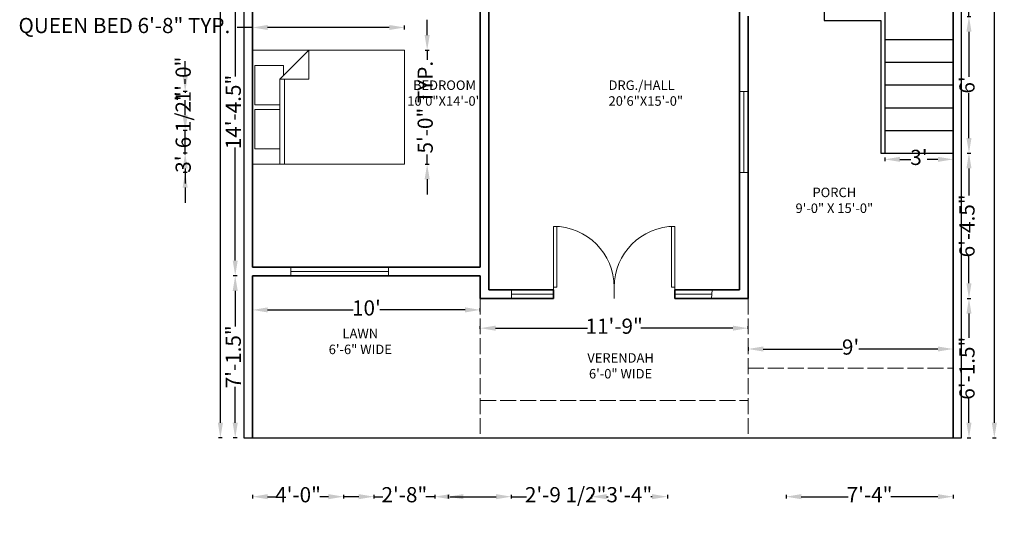
# Model space of a CAD drawing. Units: inches. Extents: x 2174 to 2692, y 577 to 1264.
# Tile 1 of 5: x 2174 to 2692, y 577 to 841. Entities that reach past the tile are written whole.
import ezdxf

# ---------------------------------------------------------------- set-up
doc = ezdxf.new("R2010")
doc.units = ezdxf.units.IN
doc.linetypes.add('ACAD_ISO02W100', pattern=[15, 12, -3])
for name, color, linetype, lineweight in [('A-ANNO-DIMS', 2, 'Continuous', 13), ('A-AREA-IDEN', 7, 'Continuous', 18), ('A-DOOR', 3, 'Continuous', 18), ('A-FLOR-EDGE', 8, 'ACAD_ISO02W100', 18), ('A-FLOR-STRS', 7, 'Continuous', 25), ('A-FURN', 8, 'Continuous', 18), ('A-GLAZ', 4, 'Continuous', 18), ('A-WALL', 7, 'Continuous', 35), ('C-PROP', 7, 'Continuous', 25)]:
    doc.layers.add(name, color=color, linetype=linetype, lineweight=lineweight)
doc.styles.get("Standard").update_dxf_attribs({"font": 'arial.ttf'})
doc.dimstyles.new('ISO-25', dxfattribs={"dimtxt": 8, "dimasz": 8, "dimexe": 1, "dimexo": 1, "dimtad": 0, "dimdec": 1, "dimlunit": 3, "dimtxsty": 'Standard', "dimcen": 2.5, "dimclrd": 1, "dimclre": 1, "dimclrt": 1, "dimadec": 0, "dimazin": 0, "dimtfac": 1, "dimtdec": 1, "dimtmove": 0, "dimatfit": 3, "dimfxl": 1, "dimfxlon": 1, "dimarcsym": 0})

# ---------------------------------------------------------------- blocks, each defined once
blk = doc.blocks.new('Bed - Queen')
for p, q in [((0, -80.00003), (0, 0)), ((0, 0), (59.99999, 0)), ((59.99999, 0), (59.99999, -80.00003)), ((7.99999, -1.2), (28.79998, -1.2)), ((7.99999, -14.4), (7.99999, -1.2)), ((28.79998, -1.2), (28.79998, -14.4)), ((31.19999, -1.2), (51.99999, -1.2)), ((31.19999, -14.4), (31.19999, -1.2)), ((51.99999, -1.2), (51.99999, -16.4)), ((0, -14.4), (44.8, -14.4)), ((59.99999, -29.6), (44.8, -14.4)), ((44.8, -14.4), (44.8, -29.6)), ((44.8, -16.8), (0, -16.8)), ((51.99999, -16.4), (46.79936, -16.4)), ((44.8, -29.6), (59.99999, -29.6)), ((59.99999, -80.00003), (0, -80.00003))]:
    blk.add_line(p, q)
blk = doc.blocks.new('*D15')
at = {"layer": 'A-ANNO-DIMS', "color": 0, "lineweight": -2, "transparency": 16777216}
for p, q in [((2629.45, 768.14), (2629.45, 766.14)), ((2665.45, 768.14), (2665.45, 766.14)), ((2637.45, 767.14), (2643.15, 767.14)), ((2657.45, 767.14), (2651.76, 767.14))]:
    blk.add_line(p, q, dxfattribs=at)
at = {"layer": 'A-ANNO-DIMS', "color": 0, "transparency": 16777216}
for points in [[(2637.45, 768.48), (2637.45, 765.81), (2629.45, 767.14)], [(2657.45, 768.48), (2657.45, 765.81), (2665.45, 767.14)]]:
    blk.add_solid(points, dxfattribs=at)
at = {"layer": 'Defpoints', "color": 0, "transparency": 16777216}
for p in [(2629.45, 770.35), (2665.45, 770.35), (2629.45, 767.14)]:
    blk.add_point(p, dxfattribs=at)
at = {"layer": 'A-ANNO-DIMS', "color": 0, "transparency": 16777216, "insert": (2647.45, 767.14), "char_height": 8, "attachment_point": 5}
blk.add_mtext("3'", dxfattribs=at)
blk = doc.blocks.new('*D16')
at = {"layer": 'A-ANNO-DIMS', "color": 0, "lineweight": -2, "transparency": 16777216}
for p, q in [((2296.45, 686.99), (2296.45, 688.82)), ((2304.45, 687.82), (2349.42, 687.82)), ((2408.45, 687.82), (2363.49, 687.82)), ((2416.45, 686.99), (2416.45, 688.82))]:
    blk.add_line(p, q, dxfattribs=at)
at = {"layer": 'A-ANNO-DIMS', "color": 0, "transparency": 16777216}
for points in [[(2304.45, 689.15), (2304.45, 686.48), (2296.45, 687.82)], [(2408.45, 689.15), (2408.45, 686.48), (2416.45, 687.82)]]:
    blk.add_solid(points, dxfattribs=at)
at = {"layer": 'Defpoints', "color": 0, "transparency": 16777216}
for p in [(2296.45, 685.99), (2416.45, 687.82), (2416.45, 685.99)]:
    blk.add_point(p, dxfattribs=at)
at = {"layer": 'A-ANNO-DIMS', "color": 0, "transparency": 16777216, "insert": (2356.45, 687.82), "char_height": 8, "attachment_point": 5}
blk.add_mtext("10'", dxfattribs=at)
blk = doc.blocks.new('*D17')
at = {"layer": 'A-ANNO-DIMS', "color": 0, "lineweight": -2, "transparency": 16777216}
for p, q in [((2416.45, 677.83), (2416.45, 679.2)), ((2424.45, 678.2), (2472.96, 678.2)), ((2549.45, 678.2), (2500.94, 678.2)), ((2557.45, 677.83), (2557.45, 679.2))]:
    blk.add_line(p, q, dxfattribs=at)
at = {"layer": 'A-ANNO-DIMS', "color": 0, "transparency": 16777216}
for points in [[(2424.45, 679.53), (2424.45, 676.87), (2416.45, 678.2)], [(2549.45, 679.53), (2549.45, 676.87), (2557.45, 678.2)]]:
    blk.add_solid(points, dxfattribs=at)
at = {"layer": 'Defpoints', "color": 0, "transparency": 16777216}
for p in [(2416.45, 676.83), (2557.45, 678.2), (2557.45, 676.83)]:
    blk.add_point(p, dxfattribs=at)
at = {"layer": 'A-ANNO-DIMS', "color": 0, "transparency": 16777216, "insert": (2486.95, 678.2), "char_height": 8, "attachment_point": 5}
blk.add_mtext('11\'-9"', dxfattribs=at)
blk = doc.blocks.new('*D18')
at = {"layer": 'A-ANNO-DIMS', "color": 0, "lineweight": -2, "transparency": 16777216}
for p, q in [((2557.45, 668.21), (2557.45, 666.21)), ((2565.45, 667.21), (2607.15, 667.21)), ((2657.45, 667.21), (2615.76, 667.21)), ((2665.45, 668.21), (2665.45, 666.21))]:
    blk.add_line(p, q, dxfattribs=at)
at = {"layer": 'A-ANNO-DIMS', "color": 0, "transparency": 16777216}
for points in [[(2565.45, 668.54), (2565.45, 665.88), (2557.45, 667.21)], [(2657.45, 668.54), (2657.45, 665.88), (2665.45, 667.21)]]:
    blk.add_solid(points, dxfattribs=at)
at = {"layer": 'Defpoints', "color": 0, "transparency": 16777216}
for p in [(2557.45, 670.41), (2665.45, 670.41), (2665.45, 667.21)]:
    blk.add_point(p, dxfattribs=at)
at = {"layer": 'A-ANNO-DIMS', "color": 0, "transparency": 16777216, "insert": (2611.45, 667.21), "char_height": 8, "attachment_point": 5}
blk.add_mtext("9'", dxfattribs=at)
blk = doc.blocks.new('*U21')
for p, q in [((0, 0), (0, -6)), ((-32, 0), (-32, -6))]:
    blk.add_line(p, q)
blk.add_lwpolyline([(0, 0), (0, 32), (-1.75, 32), (-1.75, 0)], close=True)
blk.add_arc((0, 0), 32, 90, 180)
blk = doc.blocks.new('*U22')
for p, q in [((0, 0), (0, -6)), ((32, 0), (32, -6))]:
    blk.add_line(p, q)
blk.add_lwpolyline([(0, 0), (0, 32), (1.75, 32), (1.75, 0)], close=True)
blk.add_arc((0, 0), 32, 0, 90)
blk = doc.blocks.new('*D33')
at = {"layer": 'A-ANNO-DIMS', "color": 0, "lineweight": -2, "transparency": 16777216}
for p, q in [((2288.37, 878.35), (2286.37, 878.35)), ((2287.37, 870.35), (2287.37, 810.75)), ((2287.37, 713.85), (2287.37, 773.45)), ((2288.37, 705.85), (2286.37, 705.85))]:
    blk.add_line(p, q, dxfattribs=at)
at = {"layer": 'A-ANNO-DIMS', "color": 0, "transparency": 16777216}
for points in [[(2286.03, 870.35), (2288.7, 870.35), (2287.37, 878.35)], [(2286.03, 713.85), (2288.7, 713.85), (2287.37, 705.85)]]:
    blk.add_solid(points, dxfattribs=at)
at = {"layer": 'Defpoints', "color": 0, "transparency": 16777216}
for p in [(2296.45, 878.35), (2287.37, 705.85), (2296.45, 705.85)]:
    blk.add_point(p, dxfattribs=at)
at = {"layer": 'A-ANNO-DIMS', "color": 0, "transparency": 16777216, "insert": (2287.37, 792.1), "char_height": 8, "attachment_point": 5, "rotation": 90}
blk.add_mtext('14\'-4.5"', dxfattribs=at)
blk = doc.blocks.new('*D34')
at = {"layer": 'A-ANNO-DIMS', "color": 0, "lineweight": -2, "transparency": 16777216}
for p, q in [((2288.37, 705.85), (2286.37, 705.85)), ((2287.37, 697.85), (2287.37, 678.99)), ((2287.37, 628.35), (2287.37, 647.22)), ((2288.37, 620.35), (2286.37, 620.35))]:
    blk.add_line(p, q, dxfattribs=at)
at = {"layer": 'A-ANNO-DIMS', "color": 0, "transparency": 16777216}
for points in [[(2286.03, 697.85), (2288.7, 697.85), (2287.37, 705.85)], [(2286.03, 628.35), (2288.7, 628.35), (2287.37, 620.35)]]:
    blk.add_solid(points, dxfattribs=at)
at = {"layer": 'Defpoints', "color": 0, "transparency": 16777216}
for p in [(2296.45, 705.85), (2287.37, 620.35), (2296.45, 620.35)]:
    blk.add_point(p, dxfattribs=at)
at = {"layer": 'A-ANNO-DIMS', "color": 0, "transparency": 16777216, "insert": (2287.37, 663.1), "char_height": 8, "attachment_point": 5, "rotation": 90}
blk.add_mtext('7\'-1.5"', dxfattribs=at)
blk = doc.blocks.new('*D38')
at = {"layer": 'A-ANNO-DIMS', "color": 0, "lineweight": -2, "transparency": 16777216}
for p, q in [((2673.81, 890.85), (2673.81, 898.85)), ((2672.81, 882.85), (2674.81, 882.85)), ((2673.81, 882.85), (2673.81, 878.52)), ((2673.81, 842.35), (2673.81, 846.69)), ((2672.81, 842.35), (2674.81, 842.35)), ((2673.81, 834.35), (2673.81, 826.35))]:
    blk.add_line(p, q, dxfattribs=at)
at = {"layer": 'A-ANNO-DIMS', "color": 0, "transparency": 16777216}
for points in [[(2672.48, 890.85), (2675.15, 890.85), (2673.81, 882.85)], [(2672.48, 834.35), (2675.15, 834.35), (2673.81, 842.35)]]:
    blk.add_solid(points, dxfattribs=at)
at = {"layer": 'Defpoints', "color": 0, "transparency": 16777216}
for p in [(2665.45, 882.85), (2665.45, 842.35), (2673.81, 842.35)]:
    blk.add_point(p, dxfattribs=at)
at = {"layer": 'A-ANNO-DIMS', "color": 0, "transparency": 16777216, "insert": (2673.81, 862.6), "char_height": 8, "attachment_point": 5, "rotation": 90}
blk.add_mtext('3\'-4.5"', dxfattribs=at)
blk = doc.blocks.new('*D39')
at = {"layer": 'A-ANNO-DIMS', "color": 0, "lineweight": -2, "transparency": 16777216}
for p, q in [((2672.81, 842.35), (2674.81, 842.35)), ((2673.81, 834.35), (2673.81, 810.68)), ((2673.81, 778.35), (2673.81, 802.02)), ((2672.81, 770.35), (2674.81, 770.35))]:
    blk.add_line(p, q, dxfattribs=at)
at = {"layer": 'A-ANNO-DIMS', "color": 0, "transparency": 16777216}
for points in [[(2672.48, 834.35), (2675.15, 834.35), (2673.81, 842.35)], [(2672.48, 778.35), (2675.15, 778.35), (2673.81, 770.35)]]:
    blk.add_solid(points, dxfattribs=at)
at = {"layer": 'Defpoints', "color": 0, "transparency": 16777216}
for p in [(2665.45, 842.35), (2665.45, 770.35), (2673.81, 770.35)]:
    blk.add_point(p, dxfattribs=at)
at = {"layer": 'A-ANNO-DIMS', "color": 0, "transparency": 16777216, "insert": (2673.81, 806.35), "char_height": 8, "attachment_point": 5, "rotation": 90}
blk.add_mtext("6'", dxfattribs=at)
blk = doc.blocks.new('*D40')
at = {"layer": 'A-ANNO-DIMS', "color": 0, "lineweight": -2, "transparency": 16777216}
for p, q in [((2672.81, 770.35), (2674.81, 770.35)), ((2673.81, 762.35), (2673.81, 748.04)), ((2673.81, 701.85), (2673.81, 716.16)), ((2672.81, 693.85), (2674.81, 693.85))]:
    blk.add_line(p, q, dxfattribs=at)
at = {"layer": 'A-ANNO-DIMS', "color": 0, "transparency": 16777216}
for points in [[(2672.48, 762.35), (2675.15, 762.35), (2673.81, 770.35)], [(2672.48, 701.85), (2675.15, 701.85), (2673.81, 693.85)]]:
    blk.add_solid(points, dxfattribs=at)
at = {"layer": 'Defpoints', "color": 0, "transparency": 16777216}
for p in [(2665.45, 770.35), (2557.45, 693.85), (2673.81, 693.85)]:
    blk.add_point(p, dxfattribs=at)
at = {"layer": 'A-ANNO-DIMS', "color": 0, "transparency": 16777216, "insert": (2673.81, 732.1), "char_height": 8, "attachment_point": 5, "rotation": 90}
blk.add_mtext('6\'-4.5"', dxfattribs=at)
blk = doc.blocks.new('*D41')
at = {"layer": 'A-ANNO-DIMS', "color": 0, "lineweight": -2, "transparency": 16777216}
for p, q in [((2672.81, 693.85), (2674.81, 693.85)), ((2673.81, 685.85), (2673.81, 673.04)), ((2673.81, 628.35), (2673.81, 641.16)), ((2672.81, 620.35), (2674.81, 620.35))]:
    blk.add_line(p, q, dxfattribs=at)
at = {"layer": 'A-ANNO-DIMS', "color": 0, "transparency": 16777216}
for points in [[(2672.48, 685.85), (2675.15, 685.85), (2673.81, 693.85)], [(2672.48, 628.35), (2675.15, 628.35), (2673.81, 620.35)]]:
    blk.add_solid(points, dxfattribs=at)
at = {"layer": 'Defpoints', "color": 0, "transparency": 16777216}
for p in [(2557.45, 693.85), (2669.95, 620.35), (2673.81, 620.35)]:
    blk.add_point(p, dxfattribs=at)
at = {"layer": 'A-ANNO-DIMS', "color": 0, "transparency": 16777216, "insert": (2673.81, 657.1), "char_height": 8, "attachment_point": 5, "rotation": 90}
blk.add_mtext('6\'-1.5"', dxfattribs=at)
blk = doc.blocks.new('*D42')
at = {"layer": 'A-ANNO-DIMS', "color": 0, "lineweight": -2, "transparency": 16777216}
for p, q in [((2686.18, 1220.35), (2688.18, 1220.35)), ((2687.18, 1212.35), (2687.18, 927.77)), ((2687.18, 628.35), (2687.18, 912.94)), ((2686.18, 620.35), (2688.18, 620.35))]:
    blk.add_line(p, q, dxfattribs=at)
at = {"layer": 'A-ANNO-DIMS', "color": 0, "transparency": 16777216}
for points in [[(2685.84, 1212.35), (2688.51, 1212.35), (2687.18, 1220.35)], [(2685.84, 628.35), (2688.51, 628.35), (2687.18, 620.35)]]:
    blk.add_solid(points, dxfattribs=at)
at = {"layer": 'Defpoints', "color": 0, "transparency": 16777216}
for p in [(2669.95, 1220.35), (2687.18, 1220.35), (2669.95, 620.35)]:
    blk.add_point(p, dxfattribs=at)
at = {"layer": 'A-ANNO-DIMS', "color": 0, "transparency": 16777216, "insert": (2687.18, 920.35), "char_height": 8, "attachment_point": 5, "rotation": 90}
blk.add_mtext("50'", dxfattribs=at)
blk = doc.blocks.new('*D43')
at = {"layer": 'A-ANNO-DIMS', "color": 0, "lineweight": -2, "transparency": 16777216}
for p, q in [((2280.55, 1220.35), (2278.55, 1220.35)), ((2279.55, 1212.35), (2279.55, 927.77)), ((2279.55, 628.35), (2279.55, 912.94)), ((2280.55, 620.35), (2278.55, 620.35))]:
    blk.add_line(p, q, dxfattribs=at)
at = {"layer": 'A-ANNO-DIMS', "color": 0, "transparency": 16777216}
for points in [[(2278.21, 1212.35), (2280.88, 1212.35), (2279.55, 1220.35)], [(2278.21, 628.35), (2280.88, 628.35), (2279.55, 620.35)]]:
    blk.add_solid(points, dxfattribs=at)
at = {"layer": 'Defpoints', "color": 0, "transparency": 16777216}
for p in [(2291.95, 1220.35), (2279.55, 620.35), (2291.95, 620.35)]:
    blk.add_point(p, dxfattribs=at)
at = {"layer": 'A-ANNO-DIMS', "color": 0, "transparency": 16777216, "insert": (2279.55, 920.35), "char_height": 8, "attachment_point": 5, "rotation": 90}
blk.add_mtext("50'", dxfattribs=at)
blk = doc.blocks.new('*D45')
at = {"layer": 'A-ANNO-DIMS', "color": 1, "lineweight": -2, "transparency": 16777216}
for p, q in [((2296.45, 836.64), (2288.45, 836.64)), ((2296.45, 835.64), (2296.45, 837.64)), ((2368.45, 836.64), (2304.45, 836.64)), ((2376.45, 835.64), (2376.45, 837.64))]:
    blk.add_line(p, q, dxfattribs=at)
at = {"layer": 'A-ANNO-DIMS', "color": 1, "transparency": 16777216}
for points in [[(2304.45, 837.97), (2304.45, 835.3), (2296.45, 836.64)], [(2368.45, 837.97), (2368.45, 835.3), (2376.45, 836.64)]]:
    blk.add_solid(points, dxfattribs=at)
at = {"layer": 'Defpoints', "color": 0, "transparency": 16777216}
for p in [(2296.45, 836.64), (2296.45, 824.64), (2376.45, 824.64)]:
    blk.add_point(p, dxfattribs=at)
at = {"layer": 'A-ANNO-DIMS', "color": 1, "transparency": 16777216, "insert": (2228.99, 836.64), "char_height": 8, "attachment_point": 5}
blk.add_mtext('QUEEN BED 6\'-8" TYP.', dxfattribs=at)
blk = doc.blocks.new('*D46')
at = {"layer": 'A-ANNO-DIMS', "color": 1, "lineweight": -2, "transparency": 16777216}
for p, q in [((2388.45, 832.64), (2388.45, 840.64)), ((2387.45, 824.64), (2389.45, 824.64)), ((2388.45, 824.64), (2388.45, 819.64)), ((2388.45, 764.64), (2388.45, 769.63)), ((2387.45, 764.64), (2389.45, 764.64)), ((2388.45, 756.64), (2388.45, 748.64))]:
    blk.add_line(p, q, dxfattribs=at)
at = {"layer": 'A-ANNO-DIMS', "color": 1, "transparency": 16777216}
for points in [[(2387.12, 832.64), (2389.79, 832.64), (2388.45, 824.64)], [(2387.12, 756.64), (2389.79, 756.64), (2388.45, 764.64)]]:
    blk.add_solid(points, dxfattribs=at)
at = {"layer": 'Defpoints', "color": 0, "transparency": 16777216}
for p in [(2376.45, 824.64), (2388.45, 824.64), (2376.45, 764.64)]:
    blk.add_point(p, dxfattribs=at)
at = {"layer": 'A-ANNO-DIMS', "color": 1, "transparency": 16777216, "insert": (2388.45, 794.64), "char_height": 8, "attachment_point": 5, "rotation": 90}
blk.add_mtext('5\'-0" TYP.', dxfattribs=at)
blk = doc.blocks.new('*D63')
at = {"layer": 'A-ANNO-DIMS', "color": 1, "lineweight": -2, "transparency": 16777216}
for p, q in [((2352.45, 589.4), (2344.45, 589.4)), ((2360.45, 590.4), (2360.45, 588.4)), ((2360.45, 589.4), (2365.13, 589.4)), ((2392.45, 589.4), (2387.78, 589.4)), ((2392.45, 590.4), (2392.45, 588.4)), ((2400.45, 589.4), (2408.45, 589.4))]:
    blk.add_line(p, q, dxfattribs=at)
at = {"layer": 'A-ANNO-DIMS', "color": 1, "transparency": 16777216}
for points in [[(2352.45, 590.74), (2352.45, 588.07), (2360.45, 589.4)], [(2400.45, 590.74), (2400.45, 588.07), (2392.45, 589.4)]]:
    blk.add_solid(points, dxfattribs=at)
at = {"layer": 'Defpoints', "color": 0, "transparency": 16777216}
for p in [(2360.45, 1155.85), (2392.45, 1155.6), (2392.45, 589.4)]:
    blk.add_point(p, dxfattribs=at)
at = {"layer": 'A-ANNO-DIMS', "color": 1, "transparency": 16777216, "insert": (2376.45, 589.4), "char_height": 8, "attachment_point": 5}
blk.add_mtext('2\'-8"', dxfattribs=at)
blk = doc.blocks.new('*D64')
at = {"layer": 'A-ANNO-DIMS', "color": 1, "lineweight": -2, "transparency": 16777216}
for p, q in [((2474.95, 590.4), (2474.95, 588.4)), ((2482.95, 589.4), (2483.7, 589.4)), ((2506.95, 589.4), (2506.21, 589.4)), ((2514.95, 590.4), (2514.95, 588.4))]:
    blk.add_line(p, q, dxfattribs=at)
at = {"layer": 'A-ANNO-DIMS', "color": 1, "transparency": 16777216}
for points in [[(2482.95, 590.74), (2482.95, 588.07), (2474.95, 589.4)], [(2506.95, 590.74), (2506.95, 588.07), (2514.95, 589.4)]]:
    blk.add_solid(points, dxfattribs=at)
at = {"layer": 'Defpoints', "color": 0, "transparency": 16777216}
for p in [(2474.95, 1014.85), (2514.95, 1014.85), (2514.95, 589.4)]:
    blk.add_point(p, dxfattribs=at)
at = {"layer": 'A-ANNO-DIMS', "color": 1, "transparency": 16777216, "insert": (2494.95, 589.4), "char_height": 8, "attachment_point": 5}
blk.add_mtext('3\'-4"', dxfattribs=at)
blk = doc.blocks.new('*D65')
at = {"layer": 'A-ANNO-DIMS', "color": 1, "lineweight": -2, "transparency": 16777216}
for p, q in [((2412.95, 1251.3), (2404.95, 1251.3)), ((2420.95, 1250.3), (2420.95, 1252.3)), ((2420.95, 1251.3), (2423.52, 1251.3)), ((2454.95, 1251.3), (2452.39, 1251.3)), ((2454.95, 1250.3), (2454.95, 1252.3)), ((2462.95, 1251.3), (2470.95, 1251.3))]:
    blk.add_line(p, q, dxfattribs=at)
at = {"layer": 'A-ANNO-DIMS', "color": 1, "transparency": 16777216}
for points in [[(2412.95, 1252.64), (2412.95, 1249.97), (2420.95, 1251.3)], [(2462.95, 1252.64), (2462.95, 1249.97), (2454.95, 1251.3)]]:
    blk.add_solid(points, dxfattribs=at)
at = {"layer": 'Defpoints', "color": 0, "transparency": 16777216}
for p in [(2454.95, 1251.3), (2420.95, 698.35), (2454.95, 698.35)]:
    blk.add_point(p, dxfattribs=at)
at = {"layer": 'A-ANNO-DIMS', "color": 1, "transparency": 16777216, "insert": (2437.95, 1251.3), "char_height": 8, "attachment_point": 5}
blk.add_mtext('2\'-10"', dxfattribs=at)
blk = doc.blocks.new('*D66')
at = {"layer": 'A-ANNO-DIMS', "color": 1, "lineweight": -2, "transparency": 16777216}
for p, q in [((2454.95, 1250.3), (2454.95, 1252.3)), ((2462.95, 1251.3), (2475.7, 1251.3)), ((2510.95, 1251.3), (2498.21, 1251.3)), ((2518.95, 1250.3), (2518.95, 1252.3))]:
    blk.add_line(p, q, dxfattribs=at)
at = {"layer": 'A-ANNO-DIMS', "color": 1, "transparency": 16777216}
for points in [[(2462.95, 1252.64), (2462.95, 1249.97), (2454.95, 1251.3)], [(2510.95, 1252.64), (2510.95, 1249.97), (2518.95, 1251.3)]]:
    blk.add_solid(points, dxfattribs=at)
at = {"layer": 'Defpoints', "color": 0, "transparency": 16777216}
for p in [(2518.95, 1251.3), (2454.95, 698.35), (2518.95, 698.35)]:
    blk.add_point(p, dxfattribs=at)
at = {"layer": 'A-ANNO-DIMS', "color": 1, "transparency": 16777216, "insert": (2486.95, 1251.3), "char_height": 8, "attachment_point": 5}
blk.add_mtext('5\'-4"', dxfattribs=at)
blk = doc.blocks.new('*D71')
at = {"layer": 'A-ANNO-DIMS', "color": 1, "lineweight": -2, "transparency": 16777216}
for p, q in [((2308.69, 1251.3), (2300.69, 1251.3)), ((2316.69, 1250.3), (2316.69, 1252.3)), ((2316.69, 1251.3), (2321.61, 1251.3)), ((2368.01, 1251.3), (2363.09, 1251.3)), ((2368.01, 1250.3), (2368.01, 1252.3)), ((2376.01, 1251.3), (2384.01, 1251.3))]:
    blk.add_line(p, q, dxfattribs=at)
at = {"layer": 'A-ANNO-DIMS', "color": 1, "transparency": 16777216}
for points in [[(2308.69, 1252.64), (2308.69, 1249.97), (2316.69, 1251.3)], [(2376.01, 1252.64), (2376.01, 1249.97), (2368.01, 1251.3)]]:
    blk.add_solid(points, dxfattribs=at)
at = {"layer": 'Defpoints', "color": 0, "transparency": 16777216}
for p in [(2368.01, 1251.3), (2316.69, 710.35), (2368.01, 710.35)]:
    blk.add_point(p, dxfattribs=at)
at = {"layer": 'A-ANNO-DIMS', "color": 1, "transparency": 16777216, "insert": (2342.35, 1251.3), "char_height": 8, "attachment_point": 5}
blk.add_mtext('4\'-3 1/2"', dxfattribs=at)
blk = doc.blocks.new('*D72')
at = {"layer": 'A-ANNO-DIMS', "color": 1, "lineweight": -2, "transparency": 16777216}
for p, q in [((2296.45, 1250.3), (2296.45, 1252.3)), ((2304.45, 1251.3), (2308.69, 1251.3)), ((2316.69, 1250.3), (2316.69, 1252.3)), ((2316.69, 1251.3), (2324.69, 1251.3))]:
    blk.add_line(p, q, dxfattribs=at)
at = {"layer": 'A-ANNO-DIMS', "color": 1, "transparency": 16777216}
for points in [[(2304.45, 1252.64), (2304.45, 1249.97), (2296.45, 1251.3)], [(2308.69, 1252.64), (2308.69, 1249.97), (2316.69, 1251.3)]]:
    blk.add_solid(points, dxfattribs=at)
at = {"layer": 'Defpoints', "color": 0, "transparency": 16777216}
for p in [(2316.69, 1251.3), (2296.45, 710.35), (2316.69, 710.35)]:
    blk.add_point(p, dxfattribs=at)
at = {"layer": 'A-ANNO-DIMS', "color": 1, "transparency": 16777216, "insert": (2335.57, 1251.3), "char_height": 8, "attachment_point": 5}
blk.add_mtext('1\'-8"', dxfattribs=at)
blk = doc.blocks.new('*D73')
at = {"layer": 'A-ANNO-DIMS', "color": 1, "lineweight": -2, "transparency": 16777216}
for p, q in [((2261, 810.89), (2261, 818.89)), ((2262, 802.89), (2260, 802.89)), ((2261, 802.89), (2261, 802.14)), ((2262, 760.23), (2260, 760.23)), ((2261, 760.23), (2261, 760.99)), ((2261, 752.23), (2261, 744.23))]:
    blk.add_line(p, q, dxfattribs=at)
at = {"layer": 'A-ANNO-DIMS', "color": 1, "transparency": 16777216}
for points in [[(2259.67, 810.89), (2262.34, 810.89), (2261, 802.89)], [(2259.67, 752.23), (2262.34, 752.23), (2261, 760.23)]]:
    blk.add_solid(points, dxfattribs=at)
at = {"layer": 'Defpoints', "color": 0, "transparency": 16777216}
for p in [(2261, 802.89), (2552.95, 802.89), (2552.95, 760.23)]:
    blk.add_point(p, dxfattribs=at)
at = {"layer": 'A-ANNO-DIMS', "color": 1, "transparency": 16777216, "insert": (2261, 781.56), "char_height": 8, "attachment_point": 5, "rotation": 90}
blk.add_mtext('3\'-6 1/2"', dxfattribs=at)
blk = doc.blocks.new('*D75')
at = {"layer": 'A-ANNO-DIMS', "color": 1, "lineweight": -2, "transparency": 16777216}
for p, q in [((2296.45, 590.4), (2296.45, 588.4)), ((2304.45, 589.4), (2309.03, 589.4)), ((2336.45, 589.4), (2331.87, 589.4)), ((2344.45, 590.4), (2344.45, 588.4))]:
    blk.add_line(p, q, dxfattribs=at)
at = {"layer": 'A-ANNO-DIMS', "color": 1, "transparency": 16777216}
for points in [[(2304.45, 590.74), (2304.45, 588.07), (2296.45, 589.4)], [(2336.45, 590.74), (2336.45, 588.07), (2344.45, 589.4)]]:
    blk.add_solid(points, dxfattribs=at)
at = {"layer": 'Defpoints', "color": 0, "transparency": 16777216}
for p in [(2296.45, 1014.85), (2344.45, 1014.85), (2344.45, 589.4)]:
    blk.add_point(p, dxfattribs=at)
at = {"layer": 'A-ANNO-DIMS', "color": 1, "transparency": 16777216, "insert": (2320.45, 589.4), "char_height": 8, "attachment_point": 5}
blk.add_mtext('4\'-0"', dxfattribs=at)
blk = doc.blocks.new('*D77')
at = {"layer": 'A-ANNO-DIMS', "color": 1, "lineweight": -2, "transparency": 16777216}
for p, q in [((2261, 790.35), (2261, 798.35)), ((2262, 782.35), (2260, 782.35)), ((2261, 770.35), (2261, 782.35)), ((2262, 770.35), (2260, 770.35)), ((2261, 762.35), (2261, 754.35))]:
    blk.add_line(p, q, dxfattribs=at)
at = {"layer": 'A-ANNO-DIMS', "color": 1, "transparency": 16777216}
for points in [[(2259.67, 790.35), (2262.34, 790.35), (2261, 782.35)], [(2259.67, 762.35), (2262.34, 762.35), (2261, 770.35)]]:
    blk.add_solid(points, dxfattribs=at)
at = {"layer": 'Defpoints', "color": 0, "transparency": 16777216}
for p in [(2261, 782.35), (2629.45, 782.35), (2629.45, 770.35)]:
    blk.add_point(p, dxfattribs=at)
at = {"layer": 'A-ANNO-DIMS', "color": 1, "transparency": 16777216, "insert": (2261, 809.23), "char_height": 8, "attachment_point": 5, "rotation": 90}
blk.add_mtext('1\'-0"', dxfattribs=at)
blk = doc.blocks.new('*D78')
at = {"layer": 'A-ANNO-DIMS', "color": 1, "lineweight": -2, "transparency": 16777216}
for p, q in [((2399.49, 590.4), (2399.49, 588.4)), ((2407.49, 589.4), (2424.76, 589.4)), ((2432.76, 590.4), (2432.76, 588.4)), ((2432.76, 589.4), (2440.76, 589.4))]:
    blk.add_line(p, q, dxfattribs=at)
at = {"layer": 'A-ANNO-DIMS', "color": 1, "transparency": 16777216}
for points in [[(2407.49, 590.74), (2407.49, 588.07), (2399.49, 589.4)], [(2424.76, 590.74), (2424.76, 588.07), (2432.76, 589.4)]]:
    blk.add_solid(points, dxfattribs=at)
at = {"layer": 'Defpoints', "color": 0, "transparency": 16777216}
for p in [(2399.49, 1151.35), (2432.76, 1151.35), (2432.76, 589.4)]:
    blk.add_point(p, dxfattribs=at)
at = {"layer": 'A-ANNO-DIMS', "color": 1, "transparency": 16777216, "insert": (2461.41, 589.4), "char_height": 8, "attachment_point": 5}
blk.add_mtext('2\'-9 1/2"', dxfattribs=at)
blk = doc.blocks.new('*D80')
at = {"layer": 'A-ANNO-DIMS', "color": 1, "lineweight": -2, "transparency": 16777216}
for p, q in [((2577.45, 590.4), (2577.45, 588.4)), ((2585.45, 589.4), (2610.23, 589.4)), ((2657.45, 589.4), (2632.68, 589.4)), ((2665.45, 590.4), (2665.45, 588.4))]:
    blk.add_line(p, q, dxfattribs=at)
at = {"layer": 'A-ANNO-DIMS', "color": 1, "transparency": 16777216}
for points in [[(2585.45, 590.74), (2585.45, 588.07), (2577.45, 589.4)], [(2657.45, 590.74), (2657.45, 588.07), (2665.45, 589.4)]]:
    blk.add_solid(points, dxfattribs=at)
at = {"layer": 'Defpoints', "color": 0, "transparency": 16777216}
for p in [(2577.45, 1215.85), (2665.45, 1215.85), (2665.45, 589.4)]:
    blk.add_point(p, dxfattribs=at)
at = {"layer": 'A-ANNO-DIMS', "color": 1, "transparency": 16777216, "insert": (2621.45, 589.4), "char_height": 8, "attachment_point": 5}
blk.add_mtext('7\'-4"', dxfattribs=at)

msp = doc.modelspace()

# ---------------------------------------------------------------- linework, layer by layer
at = {"layer": 'A-FLOR-EDGE', "ltscale": 0.7}
for p, q in [((2416.45, 693.85), (2416.45, 620.35)), ((2557.45, 693.85), (2557.45, 620.35)), ((2557.45, 657.1), (2665.45, 657.1)), ((2416.45, 640.02), (2557.45, 640.02))]:
    msp.add_line(p, q, dxfattribs=at)
at = {"layer": 'A-FLOR-STRS'}
for p, q in [((2597.63, 878.35), (2597.63, 840.35)), ((2629.45, 878.35), (2629.45, 840.35)), ((2597.63, 840.35), (2627.45, 840.35)), ((2627.45, 840.35), (2627.45, 770.35)), ((2629.45, 840.35), (2629.45, 770.35)), ((2629.45, 830.35), (2665.45, 830.35)), ((2629.45, 818.35), (2665.45, 818.35)), ((2629.45, 806.35), (2665.45, 806.35)), ((2629.45, 794.35), (2665.45, 794.35)), ((2629.45, 782.35), (2665.45, 782.35)), ((2627.45, 770.35), (2665.45, 770.35))]:
    msp.add_line(p, q, dxfattribs=at)
at = {"layer": 'A-GLAZ'}
for p, q in [((2552.95, 802.89), (2557.45, 802.89)), ((2555.2, 802.89), (2555.2, 760.23)), ((2552.95, 760.23), (2557.45, 760.23)), ((2316.69, 705.85), (2316.69, 710.35)), ((2316.69, 708.1), (2368.01, 708.1)), ((2368.01, 710.35), (2368.01, 705.85)), ((2432.83, 698.35), (2432.83, 693.85)), ((2432.83, 696.1), (2454.95, 696.1)), ((2538.35, 696.1), (2518.95, 696.1)), ((2538.49, 698.35), (2538.2, 693.85))]:
    msp.add_line(p, q, dxfattribs=at)
at = {"layer": 'A-WALL'}
for p, q in [((2296.45, 878.35), (2296.45, 710.35)), ((2416.45, 878.35), (2416.45, 710.35)), ((2420.95, 878.35), (2420.95, 698.35)), ((2552.95, 698.35), (2552.95, 878.35)), ((2665.45, 698.35), (2665.45, 878.35)), ((2557.45, 693.85), (2557.45, 842.61)), ((2416.45, 710.35), (2296.45, 710.35)), ((2296.45, 705.85), (2296.45, 620.35)), ((2416.45, 705.85), (2296.45, 705.85)), ((2416.45, 705.85), (2416.45, 693.85)), ((2454.95, 698.35), (2420.95, 698.35)), ((2454.95, 698.35), (2454.95, 693.85)), ((2552.95, 698.35), (2518.95, 698.35)), ((2518.95, 698.35), (2518.95, 693.85)), ((2665.45, 620.35), (2665.45, 698.35)), ((2454.95, 693.85), (2416.45, 693.85)), ((2557.45, 693.85), (2518.95, 693.85))]:
    msp.add_line(p, q, dxfattribs=at)
at = {"layer": 'C-PROP'}
for p, q in [((2291.95, 1220.35), (2291.95, 620.35)), ((2669.95, 620.35), (2669.95, 1220.35)), ((2291.95, 620.35), (2669.95, 620.35))]:
    msp.add_line(p, q, dxfattribs=at)

# ---------------------------------------------------------------- block references
at = {"layer": 'A-DOOR'}
for name, p in [('*U22', (2454.95, 699.85)), ('*U21', (2518.95, 699.85))]:
    msp.add_blockref(name, p, dxfattribs=at)
at = {"layer": 'A-FURN', "rotation": 90.0000000000235}
msp.add_blockref('Bed - Queen', (2296.45, 764.64), dxfattribs=at)

# ---------------------------------------------------------------- texts
at = {"layer": 'A-AREA-IDEN', "char_height": 5, "attachment_point": 1}
for s, width, insert in [('DRG./HALL\\P20\'6"X15\'-0"', 38.1431, (2483.98, 808.73)), ('\\pxqc;BEDROOM\\P10\'0"X14\'-0"', 38.1431, (2378.52, 808.73)), ('\\pxqc;PORCH\\P9\'-0" X 15\'-0"', 44.8921, (2580.45, 752.23)), ('\\pxqc;LAWN\\P6\'-6" WIDE', 38.1431, (2334.17, 677.85)), ('\\pxqc;VERENDAH\\P6\'-0" WIDE', 38.1431, (2471.25, 665.02))]:
    msp.add_mtext_dynamic_manual_height_columns(s, width=width, gutter_width=12.5, heights=[0], dxfattribs=dict(at, insert=insert))

# ---------------------------------------------------------------- dimensions: what is measured, and where the dimension line sits
at = {"layer": 'A-ANNO-DIMS'}
for base, p1, p2, override, picture, middle in [((2368.01, 1251.3), (2316.69, 710.35), (2368.01, 710.35), {"dimdec": 1, "dimlfac": 1, "dimrnd": 0, "dimzin": 1, "dimdsep": 46, "dimlunit": 4, "dimfrac": 2}, '*D71', (2342.35, 1251.3)), ((2316.69, 1251.3), (2296.45, 710.35), (2316.69, 710.35), {"dimdec": 1, "dimlfac": 1, "dimrnd": 0, "dimzin": 1, "dimdsep": 46, "dimlunit": 4, "dimfrac": 2}, '*D72', (2335.57, 1251.3)), ((2454.95, 1251.3), (2420.95, 698.35), (2454.95, 698.35), {"dimdec": 1, "dimlfac": 1, "dimrnd": 0, "dimzin": 1, "dimdsep": 46, "dimlunit": 4, "dimfrac": 2}, '*D65', (2437.95, 1251.3)), ((2518.95, 1251.3), (2454.95, 698.35), (2518.95, 698.35), {"dimdec": 1, "dimlfac": 1, "dimrnd": 0, "dimzin": 1, "dimdsep": 46, "dimlunit": 4, "dimfrac": 2}, '*D66', (2486.95, 1251.3)), ((2665.45, 589.4), (2577.45, 1215.85), (2665.45, 1215.85), {"dimdec": 1, "dimlfac": 1, "dimrnd": 0, "dimzin": 1, "dimdsep": 46, "dimlunit": 4, "dimfrac": 2}, '*D80', (2621.45, 589.4)), ((2392.45, 589.4), (2360.45, 1155.85), (2392.45, 1155.6), {"dimdec": 1, "dimlfac": 1, "dimrnd": 0, "dimzin": 1, "dimdsep": 46, "dimlunit": 4, "dimfrac": 2}, '*D63', (2376.45, 589.4)), ((2432.76, 589.4), (2399.49, 1151.35), (2432.76, 1151.35), {"dimdec": 1, "dimlfac": 1, "dimrnd": 0, "dimzin": 1, "dimdsep": 46, "dimlunit": 4, "dimfrac": 2}, '*D78', (2461.41, 589.4)), ((2344.45, 589.4), (2296.45, 1014.85), (2344.45, 1014.85), {"dimdec": 1, "dimlfac": 1, "dimrnd": 0, "dimzin": 1, "dimdsep": 46, "dimlunit": 4, "dimfrac": 2}, '*D75', (2320.45, 589.4)), ((2514.95, 589.4), (2474.95, 1014.85), (2514.95, 1014.85), {"dimdec": 1, "dimlfac": 1, "dimrnd": 0, "dimzin": 1, "dimdsep": 46, "dimlunit": 4, "dimfrac": 2}, '*D64', (2494.95, 589.4)), ((2629.45, 767.14), (2665.45, 770.35), (2629.45, 770.35), {"dimclrd": 0, "dimclre": 0, "dimclrt": 0}, '*D15', (2647.45, 767.14)), ((2416.45, 687.82), (2296.45, 685.99), (2416.45, 685.99), {"dimclrd": 0, "dimclre": 0, "dimclrt": 0}, '*D16', (2356.45, 687.82)), ((2557.45, 678.2), (2416.45, 676.83), (2557.45, 676.83), {"dimclrd": 0, "dimclre": 0, "dimclrt": 0}, '*D17', (2486.95, 678.2)), ((2665.45, 667.21), (2557.45, 670.41), (2665.45, 670.41), {"dimclrd": 0, "dimclre": 0, "dimclrt": 0}, '*D18', (2611.45, 667.21))]:
    dim = msp.add_linear_dim(base=base, p1=p1, p2=p2, dimstyle='ISO-25', override=override, dxfattribs=at)
    dim.commit()
    dim.dimension.update_dxf_attribs({"geometry": picture, "text_midpoint": middle})
for base, p1, p2, override, picture, middle in [((2279.55, 620.35), (2291.95, 1220.35), (2291.95, 620.35), {"dimclrd": 0, "dimclre": 0, "dimclrt": 0}, '*D43', (2279.55, 920.35)), ((2687.18, 1220.35), (2669.95, 620.35), (2669.95, 1220.35), {"dimclrd": 0, "dimclre": 0, "dimclrt": 0}, '*D42', (2687.18, 920.35)), ((2673.81, 842.35), (2665.45, 882.85), (2665.45, 842.35), {"dimclrd": 0, "dimclre": 0, "dimclrt": 0, "dimtmove": 1}, '*D38', (2673.81, 862.6)), ((2287.37, 705.85), (2296.45, 878.35), (2296.45, 705.85), {"dimclrd": 0, "dimclre": 0, "dimclrt": 0, "dimtmove": 1}, '*D33', (2287.37, 792.1)), ((2673.81, 770.35), (2665.45, 842.35), (2665.45, 770.35), {"dimclrd": 0, "dimclre": 0, "dimclrt": 0, "dimtmove": 1}, '*D39', (2673.81, 806.35)), ((2261, 782.35), (2629.45, 770.35), (2629.45, 782.35), {"dimdec": 1, "dimlfac": 1, "dimrnd": 0, "dimzin": 1, "dimdsep": 46, "dimlunit": 4, "dimfrac": 2}, '*D77', (2261, 809.23)), ((2261, 802.89), (2552.95, 760.23), (2552.95, 802.89), {"dimdec": 1, "dimlfac": 1, "dimrnd": 0, "dimzin": 1, "dimdsep": 46, "dimlunit": 4, "dimfrac": 2}, '*D73', (2261, 781.56)), ((2673.81, 693.85), (2665.45, 770.35), (2557.45, 693.85), {"dimclrd": 0, "dimclre": 0, "dimclrt": 0, "dimtmove": 1}, '*D40', (2673.81, 732.1)), ((2287.37, 620.35), (2296.45, 705.85), (2296.45, 620.35), {"dimclrd": 0, "dimclre": 0, "dimclrt": 0, "dimtmove": 1}, '*D34', (2287.37, 663.1)), ((2673.81, 620.35), (2557.45, 693.85), (2669.95, 620.35), {"dimclrd": 0, "dimclre": 0, "dimclrt": 0, "dimtmove": 1}, '*D41', (2673.81, 657.1))]:
    dim = msp.add_linear_dim(base=base, p1=p1, p2=p2, angle=90, dimstyle='ISO-25', override=override, dxfattribs=at)
    dim.commit()
    dim.dimension.update_dxf_attribs({"geometry": picture, "text_midpoint": middle})
for base, p1, p2, angle, text, picture, middle in [((2296.45, 836.64), (2376.45, 824.64), (2296.45, 824.64), 180, 'QUEEN BED <> TYP.', '*D45', (2228.99, 836.64)), ((2388.45, 824.64), (2376.45, 764.64), (2376.45, 824.64), 90, '<> TYP.', '*D46', (2388.45, 794.64))]:
    dim = msp.add_linear_dim(base=base, p1=p1, p2=p2, angle=angle, text=text, dimstyle='ISO-25', override={"dimdec": 1, "dimlfac": 1, "dimrnd": 0, "dimzin": 1, "dimdsep": 46, "dimlunit": 4, "dimfrac": 2}, dxfattribs=at)
    dim.commit()
    dim.dimension.update_dxf_attribs({"geometry": picture, "text_midpoint": middle})

doc.saveas('drawing.dxf')
